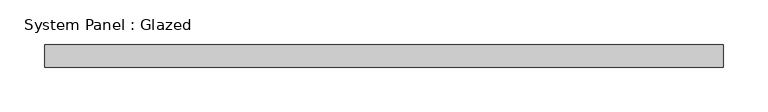
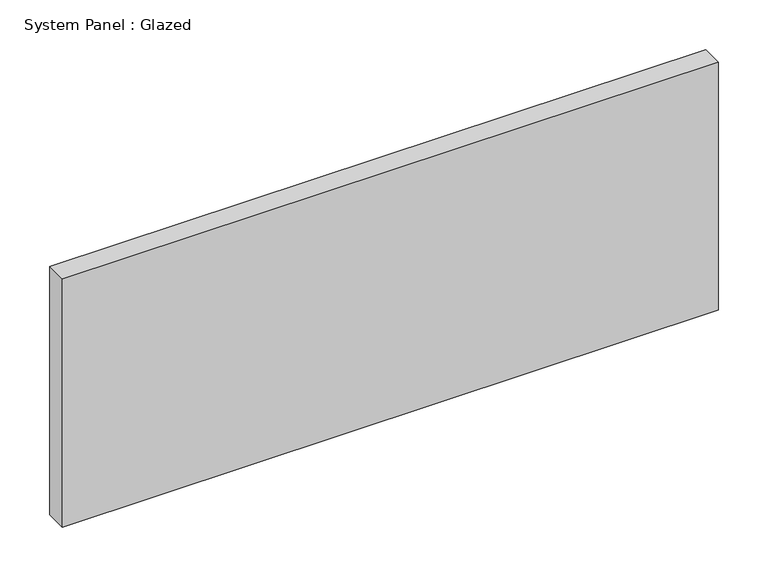
"""IFC4 building model written with IfcOpenShell, lengths in millimetres: plate geometry, System Panel : Glazed."""

from ifc_helpers import new_model, si_unit, origin, origin_with_axes, place, context, project, spatial, polyline, outline, extrude, source, transform, mapped, element, save


def system_panel_glazed_074527c7(model_context):
    return source(origin(), model_context, "Body", "SweptSolid", [
        extrude(outline(polyline([(381.0, 19.05), (-381.0, 19.05), (-381.0, 44.45), (381.0, 44.45), (381.0, 19.05)])), origin_with_axes(), (0.0, 0.0, 1.0), 304.8),
    ])


if __name__ == "__main__":
    model = new_model("IFC4")
    model_context = context("Model", 3, world=origin())
    ifc_project = project(units=[si_unit("LENGTHUNIT", "METRE", prefix="MILLI")], contexts=[model_context])
    site = spatial("IfcSite", under=ifc_project)
    building = spatial("IfcBuilding", under=site)
    placement = place(None, origin())
    system_panel_glazed_shape = system_panel_glazed_074527c7(model_context)
    element("IfcPlate", 1, ObjectType="System Panel : Glazed", at=placement, inside=building, context=model_context, shape_type="MappedRepresentation", body=[
        mapped(system_panel_glazed_shape, transform((0.0, 0.0, 0.0), x_axis=(1.0, 0.0, 0.0), y_axis=(0.0, 1.0, 0.0), z_axis=(0.0, 0.0, 1.0))),
    ])
    save(model, "model.ifc")

# Revit data of these elements
# Type "System Panel : Glazed"
#   Construction Type Id = "GSP4R"
#   Analytic Construction = "1/8 in Pilkington single glazing"
#   Visual Light Transmittance = 0.9
#   Solar Heat Gain Coefficient = 0.86
#   Heat Transfer Coefficient (U) = 1.18115 BTU/(h·ft²·°F)
#   Define Thermal Properties by = 1
# Element 1 (IfcPlate, "System Panel : Glazed")
#   Materials on its faces: "Glass"
# Materials
#   "Glass": class "Glass", colour RGB 0 128 192, transparency 0.75, Description = "Soda Lime Glass", Cost = 0
